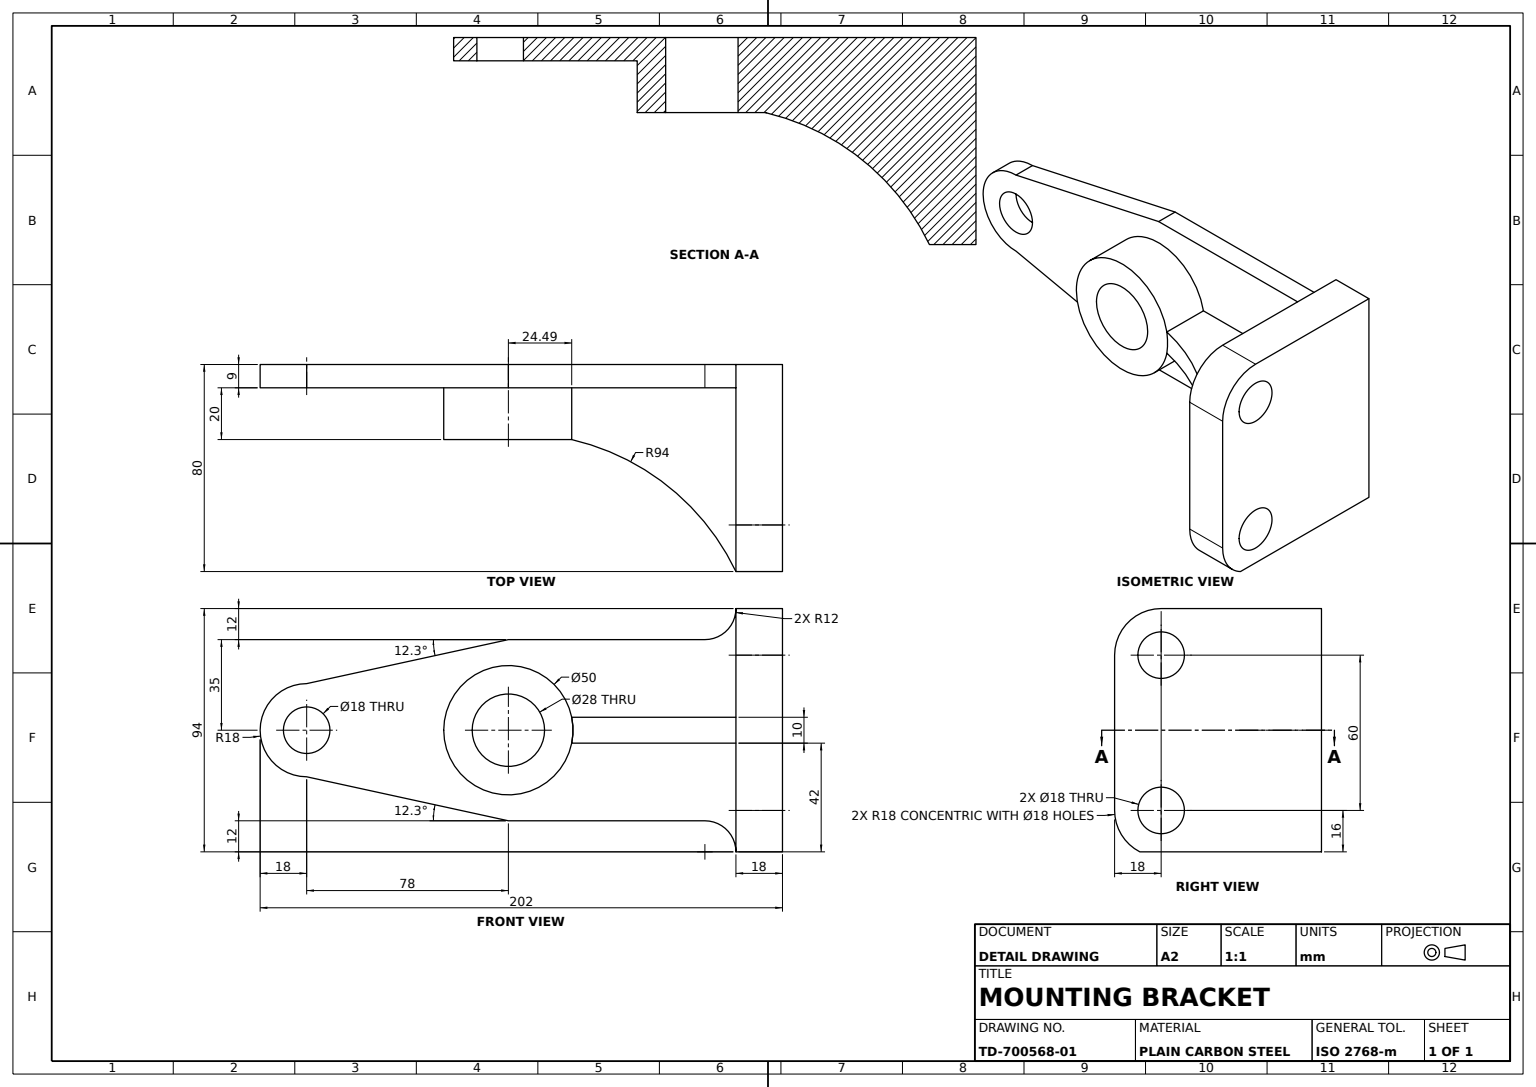
from build123d import *

# Parameters (mm, degrees)
ARM_PLATE_SKETCH_R        = 9
ARM_PLATE_SKETCH_R_2      = 14
ARM_PLATE_DEPTH           = 9
MOUNTING_FLANGE_SKETCH_R  = 9
MOUNTING_FLANGE_DEPTH     = 18
CONNECTING_BLOCK_SKETCH_W = 9
CONNECTING_BLOCK_SKETCH_H = 94
CONNECTING_BLOCK_DEPTH    = 18
HUB_BOSS_SKETCH_R         = 25
HUB_BOSS_SKETCH_R_2       = 14
HUB_BOSS_DEPTH            = 20
SUPPORT_RIB_DEPTH         = 71
PROFILE_TRIM_CUT_DEPTH    = 143.618371888
FLANGE_CUT_SKETCH_W       = 18
FLANGE_CUT_SKETCH_H       = 2
FLANGE_CUT_DEPTH          = 137.667479724


with BuildPart() as part:
    # Arm Plate Sketch → Arm Plate (new body)
    with BuildSketch(Plane.XY):
        with BuildLine():
            Line((76, 35), (0, 35))
            Line((0, 35), (-78, 18))
            ThreePointArc((-78, 18), (-96, 0), (-78, -18))
            Line((-78, -18), (0, -35))
            Line((0, -35), (76, -35))
            ThreePointArc((76, -35), (84.485281374, -38.514718626), (88, -47))
            Line((88, -47), (88, 47))
            ThreePointArc((88, 47), (84.485281374, 38.514718626), (76, 35))
        make_face()
        with Locations((-78, 0)):
            Circle(ARM_PLATE_SKETCH_R, mode=Mode.SUBTRACT)
        Circle(ARM_PLATE_SKETCH_R_2, mode=Mode.SUBTRACT)
    extrude(amount=ARM_PLATE_DEPTH)



with BuildPart() as body_2:
    # Mounting Flange Sketch → Mounting Flange (new body)
    with BuildSketch(Plane(origin=(88, 0, 0), x_dir=(0, 0, -1), z_dir=(1, 0, 0))):
        with BuildLine():
            Line((-9, 47), (-62, 47))
            ThreePointArc((-62, 47), (-74.727922061, 41.727922061), (-80, 29))
            Line((-80, 29), (-80, -31))
            ThreePointArc((-80, -31), (-74.727922061, -43.727922061), (-62, -49))
            Line((-62, -49), (-9, -49))
            Line((-9, -49), (-9, 47))
        make_face()
        with Locations((-62, 29)):
            Circle(MOUNTING_FLANGE_SKETCH_R, mode=Mode.SUBTRACT)
        with Locations((-62, -31)):
            Circle(MOUNTING_FLANGE_SKETCH_R, mode=Mode.SUBTRACT)
    extrude(amount=MOUNTING_FLANGE_DEPTH)


with BuildPart() as part_1:
    add(part.part)

    add(body_2.part)  # Connecting Block merges body 2
    # Connecting Block Sketch → Connecting Block (add)
    with BuildSketch(Plane(origin=(88, 0, 0), x_dir=(0, 0, -1), z_dir=(1, 0, 0))):
        with Locations((-4.5, 0)):
            Rectangle(CONNECTING_BLOCK_SKETCH_W, CONNECTING_BLOCK_SKETCH_H)
    extrude(amount=CONNECTING_BLOCK_DEPTH)

    # Hub Boss Sketch → Hub Boss (add)
    with BuildSketch(Plane.XY.offset(9)):
        Circle(HUB_BOSS_SKETCH_R)
        Circle(HUB_BOSS_SKETCH_R_2, mode=Mode.SUBTRACT)
    extrude(amount=HUB_BOSS_DEPTH)

    # Support Rib Sketch → Support Rib (add)
    with BuildSketch(Plane.XY.offset(9)):
        with BuildLine():
            Line((88, 0), (88, 5))
            Line((88, 5), (24.494897428, 5))
            ThreePointArc((24.494897428, 5), (24.873403825, 2.51272405), (25, 0))
            ThreePointArc((25, 0), (24.873403825, -2.51272405), (24.494897428, -5))
            Line((24.494897428, -5), (88, -5))
            Line((88, -5), (88, 0))
        make_face()
    extrude(amount=SUPPORT_RIB_DEPTH)

    # Profile Trim Cut Sketch → Profile Trim Cut (cut, through all)
    with BuildSketch(Plane.XZ.offset(5)):
        with BuildLine():
            Line((88, 80), (24.494897428, 80))
            Line((24.494897428, 80), (24.494897428, 29))
            ThreePointArc((24.494897428, 29), (62.058045644, 47.264655803), (88, 80))
        make_face()
    extrude(amount=-PROFILE_TRIM_CUT_DEPTH, mode=Mode.SUBTRACT)

    # Flange Cut Sketch → Flange Cut (cut, through all)
    with BuildSketch(Plane(origin=(0, 0, 9), x_dir=(-1, 0, 0), z_dir=(0, 0, -1))):
        with Locations((-97, -48)):
            Rectangle(FLANGE_CUT_SKETCH_W, FLANGE_CUT_SKETCH_H)
    extrude(amount=-FLANGE_CUT_DEPTH, mode=Mode.SUBTRACT)


solid = part_1.part
